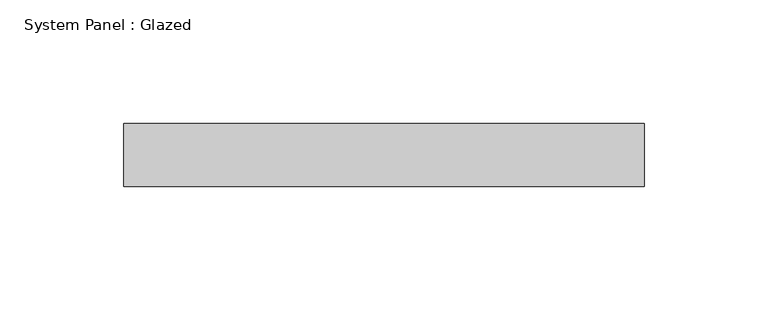
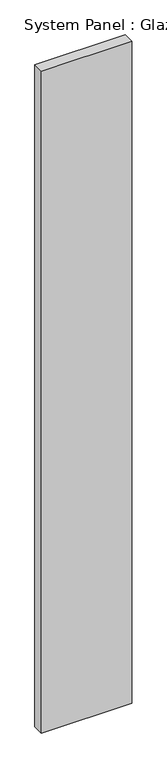
"""IFC4 building model written with IfcOpenShell, lengths in millimetres: plate geometry, System Panel : Glazed."""

from ifc_helpers import new_model, si_unit, origin, origin_with_axes, place, context, project, spatial, polyline, outline, extrude, source, transform, mapped, element, save


def system_panel_glazed_87282c25(model_context):
    return source(origin(), model_context, "Body", "SweptSolid", [
        extrude(outline(polyline([(104.9570678, 19.05), (-104.9570678, 19.05), (-104.9570678, 44.45), (104.9570678, 44.45), (104.9570678, 19.05)])), origin_with_axes(), (0.0, 0.0, 1.0), 1625.6),
    ])


if __name__ == "__main__":
    model = new_model("IFC4")
    model_context = context("Model", 3, world=origin())
    ifc_project = project(units=[si_unit("LENGTHUNIT", "METRE", prefix="MILLI")], contexts=[model_context])
    site = spatial("IfcSite", under=ifc_project)
    building = spatial("IfcBuilding", under=site)
    placement = place(None, origin())
    system_panel_glazed_shape = system_panel_glazed_87282c25(model_context)
    element("IfcPlate", 1, ObjectType="System Panel : Glazed", at=placement, inside=building, context=model_context, shape_type="MappedRepresentation", body=[
        mapped(system_panel_glazed_shape, transform((0.0, 0.0, 0.0), x_axis=(1.0, 0.0, 0.0), y_axis=(0.0, 1.0, 0.0), z_axis=(0.0, 0.0, 1.0))),
    ])
    save(model, "model.ifc")

# Revit data of these elements
# Type "System Panel : Glazed"
#   Construction Type Id = "GSP4R"
#   Analytic Construction = "1/8 in Pilkington single glazing"
#   Visual Light Transmittance = 0.9
#   Solar Heat Gain Coefficient = 0.86
#   Heat Transfer Coefficient (U) = 1.18115 BTU/(h·ft²·°F)
# Element 1 (IfcPlate, "System Panel : Glazed")
#   Materials on its faces: "Glass"
# Materials
#   "Glass": class "Glass", colour RGB 0 128 192, transparency 0.75, Description = "Soda Lime Glass", Cost = 0
